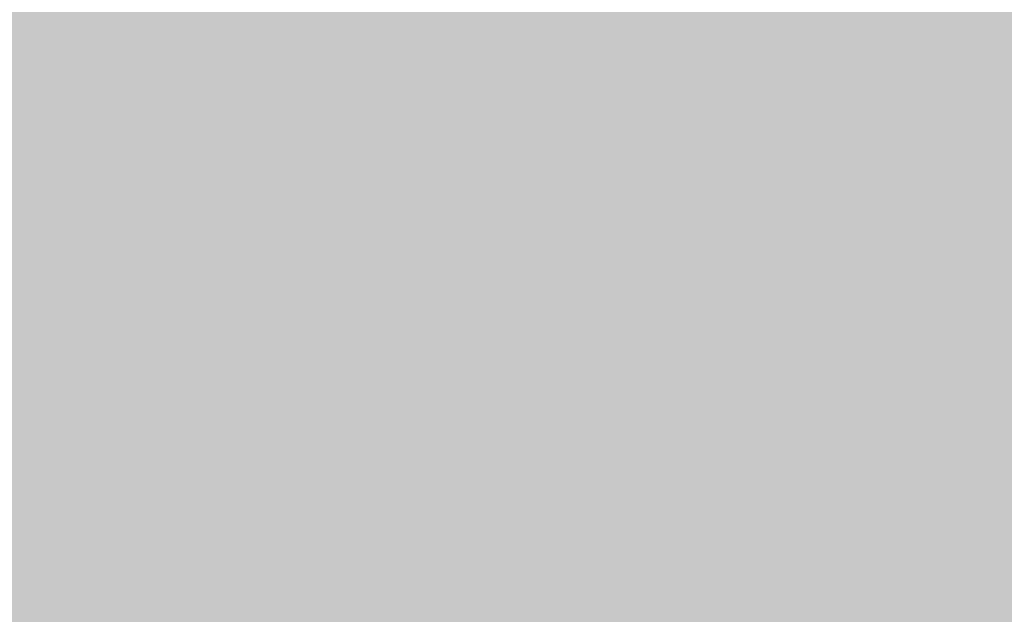
# Model space of a CAD drawing. Units: feet. Extents: x 3168 to 4724, y 827 to 1477.
# Tile 132 of 256: x 3300.858 to 3301.945, y 1098.344 to 1099.001. Entities that reach past the tile are written whole.
import ezdxf

# ---------------------------------------------------------------- set-up
doc = ezdxf.new("R2010")
doc.units = ezdxf.units.FT
doc.layers.add('A-ELEV', color=7, linetype='Continuous', lineweight=35)
doc.layers.add('A-ELEV-PATT', color=8, linetype='Continuous', lineweight=13)

msp = doc.modelspace()

# ---------------------------------------------------------------- hatches: boundary and pattern name
at = {"layer": 'A-ELEV-PATT'}
h = msp.add_hatch(color=256, dxfattribs=at)
h.dxf.hatch_style = 1
edge = h.paths.add_edge_path()
edge.add_ellipse((3552.9058, 979.2201), major_axis=(36.7449, 0), ratio=0.4848485, start_angle=0, end_angle=360)
edge = h.paths.add_edge_path()
edge.add_ellipse((3559.8916, 929.2523), major_axis=(36.7449, 0), ratio=0.4848485, start_angle=0, end_angle=360)
edge = h.paths.add_edge_path()
edge.add_line((3299.3168, 1198.6061), (3479.9167, 1198.6061))
edge.add_line((3479.9167, 1198.6061), (3479.9167, 1209.8686))
edge.add_spline(control_points=[(3479.9167, 1209.8686), (3464.3012, 1209.8686), (3448.6856, 1209.8686), (3410.9491, 1209.8686), (3388.8282, 1209.8686), (3355.6469, 1209.8686), (3344.5864, 1209.8686), (3327.9957, 1209.8686), (3322.4655, 1209.8686), (3314.1702, 1209.8686), (3311.4051, 1209.8686), (3307.2574, 1209.8686), (3305.8748, 1209.8686), (3303.801, 1209.8686), (3303.1097, 1209.8686), (3302.0728, 1209.8686), (3301.7272, 1209.8686), (3301.2087, 1209.8686), (3301.0359, 1209.8686), (3300.7767, 1209.8686), (3300.6903, 1209.8686), (3300.5606, 1209.8686), (3300.5174, 1209.8686), (3300.4526, 1209.8686), (3300.431, 1209.8686), (3300.3986, 1209.8686), (3300.3878, 1209.8686), (3300.3662, 1209.8686), (3300.3457, 1209.8686), (3300.3455, 1209.8686), (3300.3455, 1209.8686), (3300.3433, 1209.8686), (3300.3411, 1209.8686), (3300.3379, 1209.8686), (3300.3368, 1209.8686), (3300.3339, 1209.8686), (3300.3321, 1209.8686), (3300.3255, 1209.8686), (3300.3207, 1209.8686), (3300.3109, 1209.8686), (3300.306, 1209.8686), (3300.2905, 1209.8686), (3300.28, 1209.8686), (3300.2324, 1209.8688), (3300.1953, 1209.869), (3299.9511, 1209.8706), (3299.7448, 1209.8743), (3299.4368, 1209.8833), (3299.3344, 1209.8868), (3299.1811, 1209.8929), (3299.13, 1209.8951), (3298.6522, 1209.9168), (3298.2295, 1209.9457), (3297.6016, 1210.0024), (3297.3934, 1210.0235), (3297.0827, 1210.0583), (3296.9793, 1210.0705), (3296.293, 1210.1549), (3295.7181, 1210.2434), (3294.8687, 1210.3989), (3294.5877, 1210.4545), (3294.1693, 1210.5433), (3294.0304, 1210.5739), (3291.7071, 1211.1012), (3289.6536, 1211.8134), (3285.7763, 1213.564), (3283.9514, 1214.6035), (3280.5122, 1216.9801), (3278.8972, 1218.3176), (3276.3799, 1220.8295), (3275.416, 1221.9177), (3274.0393, 1223.7077), (3273.581, 1224.3495), (3273.1432, 1225.0163)], knot_values=[39.119033, 39.119033, 39.119033, 39.119033, 39.286353, 39.286353, 39.523379, 39.523379, 39.641892, 39.641892, 39.701148, 39.701148, 39.730777, 39.730777, 39.745591, 39.745591, 39.752998, 39.752998, 39.756701, 39.756701, 39.758553, 39.758553, 39.759479, 39.759479, 39.759942, 39.759942, 39.760173, 39.760173, 39.760289, 39.760289, 39.760405, 39.760405, 39.760463, 39.760463, 39.763389, 39.763389, 39.764851, 39.764851, 39.767304, 39.767304, 39.773825, 39.773825, 39.78057, 39.78057, 39.79477, 39.79477, 39.845194, 39.845194, 40.126715, 40.126715, 40.267476, 40.267476, 40.337856, 40.337856, 40.927023, 40.927023, 41.221606, 41.221606, 41.368898, 41.368898, 42.202622, 42.202622, 42.619485, 42.619485, 42.827916, 42.827916, 46.118323, 46.118323, 49.408731, 49.408731, 52.699139, 52.699139, 54.927489, 54.927489, 56.104228, 56.104228, 56.104228, 56.104228], weights=[1, 1, 1, 1, 1, 1, 1, 1, 1, 1, 1, 1, 1, 1, 1, 1, 1, 1, 1, 1, 1, 1, 1, 1, 1, 1, 1, 1, 1, 1, 1, 1, 1, 1, 1, 1, 1, 1, 1, 1, 1, 1, 1, 1, 1, 1, 1, 1, 1, 1, 1, 1, 1, 1, 1, 1, 1, 1, 1, 1, 1, 1, 1, 1, 1, 1, 1, 1, 1, 1, 1, 1, 1, 1], degree=3, periodic=0)
edge.add_line((3273.1432, 1225.0163), (3273.1432, 1099.0163))
edge.add_line((3273.1432, 1099.0163), (3299.3168, 1099.0163))
edge.add_line((3299.3168, 1099.0163), (3299.3168, 1198.6061))
edge = h.paths.add_edge_path()
edge.add_line((3304.7584, 1324.1581), (3479.9167, 1324.1581))
edge.add_line((3479.9167, 1324.1581), (3479.9167, 1335.7146))
edge.add_line((3479.9167, 1335.7146), (3269.1616, 1335.7146))
edge.add_spline(control_points=[(3269.1616, 1335.7146), (3264.0242, 1335.7146), (3258.3641, 1328.9582), (3259.2643, 1323.9003)], knot_values=[0, 0, 0, 0, 15.412191, 15.412191, 15.412191, 15.412191], degree=3, periodic=0)
edge.add_line((3259.2643, 1323.9003), (3265.5168, 1288.7691))
edge.add_line((3265.5168, 1288.7691), (3275.2651, 1261.5456))
edge.add_line((3275.2651, 1261.5456), (3304.7584, 1261.5456))
edge.add_line((3304.7584, 1261.5456), (3304.7584, 1324.1581))
h = msp.add_hatch(color=256, dxfattribs=at)
h.dxf.hatch_style = 1
h.paths.add_polyline_path([(3384.5252, 1099.0163), (3335.0292, 1099.0163), (3299.3168, 1099.0163), (3273.1432, 1099.0163), (3217.5654, 1099.0163), (3168.0693, 827.1163), (3335.0292, 827.1163)])

# ---------------------------------------------------------------- linework, layer by layer
at = {"layer": 'A-ELEV'}
msp.add_open_spline([(3808.5202, 1099.0163), (3808.5202, 1141.4132), (3808.5202, 1183.8102), (3808.5202, 1226.6353), (3808.5202, 1227.0636), (3808.5202, 1227.4918), (3811.4919, 1248.9947), (3814.4635, 1270.4975), (3817.4652, 1292.2176), (3817.4952, 1292.4348), (3817.5253, 1292.652), (3817.5728, 1310.1067), (3817.6203, 1327.5615), (3817.6679, 1345.0163), (3817.6679, 1345.458), (3817.6679, 1345.8996), (3817.6679, 1346.456), (3817.6679, 1346.5708), (3817.6679, 1346.7529), (3817.6679, 1346.8201), (3817.6679, 1346.9349), (3817.6679, 1346.9823), (3817.6679, 1347.0386), (3817.6679, 1347.0474), (3817.6679, 1347.0737), (3817.6679, 1347.0593), (3817.6679, 1347.0615), (3817.6679, 1347.0627), (3817.6679, 1347.066), (3817.6679, 1347.0683), (3817.6679, 1347.075), (3817.6679, 1347.0795), (3817.6678, 1347.0929), (3817.6678, 1347.1019), (3817.6678, 1347.1288), (3817.6677, 1347.1467), (3817.6674, 1347.2004), (3817.6672, 1347.2362), (3817.6661, 1347.3434), (3817.665, 1347.4147), (3817.6608, 1347.6281), (3817.6566, 1347.7697), (3817.64, 1348.1925), (3817.6235, 1348.4716), (3817.5591, 1349.3001), (3817.4961, 1349.8406), (3817.2554, 1351.4242), (3817.0263, 1352.4288), (3816.3069, 1354.8889), (3815.7437, 1356.2687), (3814.464, 1358.8192), (3813.7464, 1359.991), (3812.1958, 1362.1723), (3811.3622, 1363.1821), (3809.5888, 1365.069), (3808.6488, 1365.9461), (3806.6543, 1367.5796), (3805.5997, 1368.3362), (3803.3529, 1369.7223), (3802.1605, 1370.3524), (3799.6008, 1371.4536), (3798.2327, 1371.9255), (3795.2801, 1372.6346), (3793.6931, 1372.8721), (3791.8694, 1372.9265), (3791.7409, 1372.9292), (3791.3534, 1372.9341), (3791.0927, 1372.9329), (3790.3041, 1372.9151), (3789.7695, 1372.8842), (3789.2092, 1372.8302), (3789.1906, 1372.8284), (3789.1349, 1372.8229), (3789.0977, 1372.8191), (3789.0484, 1372.814), (3789.0364, 1372.8127), (3789.0003, 1372.8089), (3788.9761, 1372.8063), (3788.9494, 1372.8034), (3788.9468, 1372.8031), (3788.9426, 1372.8027), (3788.941, 1372.8025), (3788.9386, 1372.8022), (3788.9378, 1372.8021), (3788.9354, 1372.8019), (3788.8675, 1372.7944), (3788.7569, 1372.7822), (3788.7015, 1372.7761), (3788.5355, 1372.7579), (3788.4249, 1372.7457), (3788.0929, 1372.7092), (3787.8715, 1372.6848), (3787.2075, 1372.6118), (3786.7648, 1372.5631), (3785.4368, 1372.417), (3784.5515, 1372.3196), (3781.8954, 1372.0274), (3780.1247, 1371.8327), (3774.8126, 1371.2483), (3771.2713, 1370.8587), (3760.6471, 1369.69), (3753.5643, 1368.9109), (3732.316, 1366.5735), (3718.1504, 1365.0152), (3694.0068, 1362.3593), (3684.0287, 1361.2617), (3674.0506, 1360.1641), (3664.6007, 1360.1641), (3655.1508, 1360.1641), (3626.8011, 1360.1641), (3607.9013, 1360.1641), (3551.2019, 1360.1641), (3513.4023, 1360.1641), (3467.7252, 1360.1641), (3459.8476, 1360.1641), (3436.2149, 1360.1641), (3420.4597, 1360.1641), (3373.1943, 1360.1641), (3341.6839, 1360.1641), (3302.8482, 1360.1641), (3295.5227, 1360.1641), (3286.0383, 1360.1641), (3283.8794, 1360.1641), (3277.4026, 1360.1641), (3273.0848, 1360.1641), (3267.7329, 1360.1641), (3266.6988, 1360.1641), (3263.5965, 1360.1641), (3261.5284, 1360.1641), (3259.2369, 1360.1641), (3259.0137, 1360.1641), (3258.344, 1360.1641), (3257.8975, 1360.1641), (3257.431, 1360.1641), (3257.411, 1360.1641), (3257.3706, 1360.1641), (3257.3755, 1360.1641), (3257.3746, 1360.1641), (3257.3739, 1360.1641), (3257.372, 1360.1641), (3257.3706, 1360.1641), (3257.3667, 1360.1641), (3257.364, 1360.1641), (3257.3561, 1360.1641), (3257.3508, 1360.164), (3257.335, 1360.164), (3257.3244, 1360.164), (3257.2928, 1360.1639), (3257.2717, 1360.1638), (3257.2084, 1360.1634), (3257.1663, 1360.163), (3257.0402, 1360.1614), (3256.9563, 1360.1598), (3256.7055, 1360.1534), (3256.5392, 1360.147), (3256.0436, 1360.1219), (3255.7173, 1360.0971), (3254.7524, 1360.0005), (3254.128, 1359.9065), (3252.1801, 1359.5253), (3250.9416, 1359.144), (3248.6702, 1358.2433), (3247.6357, 1357.7238), (3245.7326, 1356.6035), (3244.8634, 1356.0021), (3243.2531, 1354.7429), (3242.512, 1354.0847), (3240.7511, 1352.3448), (3239.801, 1351.2296), (3238.0878, 1348.8724), (3237.3247, 1347.6304), (3235.9825, 1344.9716), (3235.4022, 1343.5549), (3234.5911, 1340.8155), (3234.3109, 1339.5435), (3233.9765, 1336.8026), (3233.9221, 1335.3309), (3234.1489, 1332.5913), (3234.3495, 1331.3672), (3234.7199, 1329.9994), (3234.7524, 1329.8834), (3234.8536, 1329.5348), (3234.9259, 1329.3017), (3235.0248, 1329.0026), (3235.0469, 1328.9369), (3235.0776, 1328.8472), (3235.0859, 1328.8232), (3235.1109, 1328.7511), (3235.1278, 1328.703), (3235.148, 1328.6462), (3235.1511, 1328.6376), (3235.1561, 1328.6235), (3235.1581, 1328.618), (3235.1602, 1328.612), (3235.1656, 1328.5969), (3235.1801, 1328.5565), (3235.1903, 1328.5281), (3235.2208, 1328.4429), (3235.2411, 1328.3862), (3235.3021, 1328.2159), (3235.3427, 1328.1023), (3235.4647, 1327.7617), (3235.546, 1327.5346), (3235.79, 1326.8534), (3235.9526, 1326.3992), (3236.4405, 1325.0367), (3236.7657, 1324.1284), (3237.7415, 1321.4034), (3238.392, 1319.5868), (3240.3435, 1314.1369), (3241.6445, 1310.5036), (3245.5476, 1299.6037), (3248.1496, 1292.3371), (3255.9557, 1270.5374), (3261.1598, 1256.0042), (3267.3876, 1238.612), (3268.4114, 1235.7529), (3269.5104, 1232.6839), (3269.5856, 1232.4739), (3269.7066, 1232.1359), (3269.7524, 1232.0079), (3269.8273, 1231.7987), (3269.8564, 1231.7176), (3269.9063, 1231.5781), (3269.9272, 1231.5198), (3269.9725, 1231.3934), (3269.9968, 1231.3254), (3270.0265, 1231.2425), (3270.0318, 1231.2277), (3270.0403, 1231.204), (3270.0392, 1231.207), (3270.0394, 1231.2066), (3270.0394, 1231.2064), (3270.0396, 1231.2058), (3270.0398, 1231.2055), (3270.0402, 1231.2043), (3270.0404, 1231.2036), (3270.0413, 1231.2013), (3270.0418, 1231.1998), (3270.0434, 1231.1953), (3270.0445, 1231.1922), (3270.0478, 1231.1832), (3270.0499, 1231.1771), (3270.0564, 1231.159), (3270.0608, 1231.147), (3270.0739, 1231.1108), (3270.0826, 1231.0867), (3270.1089, 1231.0144), (3270.1266, 1230.9663), (3270.1799, 1230.8225), (3270.2159, 1230.7269), (3270.3253, 1230.4415), (3270.4, 1230.2528), (3270.6292, 1229.6914), (3270.7889, 1229.3235), (3271.2865, 1228.2383), (3271.6431, 1227.5398), (3272.7759, 1225.5153), (3273.6142, 1224.2605), (3275.416, 1221.9177), (3276.3799, 1220.8295), (3278.8972, 1218.3176), (3280.5122, 1216.9801), (3283.9514, 1214.6035), (3285.7763, 1213.564), (3289.6536, 1211.8134), (3291.7071, 1211.1012), (3294.0304, 1210.5739), (3294.1693, 1210.5433), (3294.5877, 1210.4545), (3294.8687, 1210.3989), (3295.7181, 1210.2434), (3296.293, 1210.1549), (3296.9793, 1210.0705), (3297.0827, 1210.0583), (3297.3934, 1210.0235), (3297.6016, 1210.0024), (3298.2295, 1209.9457), (3298.6522, 1209.9168), (3299.13, 1209.8951), (3299.1811, 1209.8929), (3299.3344, 1209.8868), (3299.4368, 1209.8833), (3299.7448, 1209.8743), (3299.9511, 1209.8706), (3300.1953, 1209.869), (3300.2324, 1209.8688), (3300.28, 1209.8686), (3300.2905, 1209.8686), (3300.306, 1209.8686), (3300.3109, 1209.8686), (3300.3207, 1209.8686), (3300.3255, 1209.8686), (3300.3321, 1209.8686), (3300.3339, 1209.8686), (3300.3368, 1209.8686), (3300.3379, 1209.8686), (3300.3411, 1209.8686), (3300.3433, 1209.8686), (3300.3455, 1209.8686), (3300.3455, 1209.8686), (3300.3457, 1209.8686), (3300.3662, 1209.8686), (3300.3878, 1209.8686), (3300.3986, 1209.8686), (3300.431, 1209.8686), (3300.4526, 1209.8686), (3300.5174, 1209.8686), (3300.5606, 1209.8686), (3300.6903, 1209.8686), (3300.7767, 1209.8686), (3301.0359, 1209.8686), (3301.2087, 1209.8686), (3301.7272, 1209.8686), (3302.0728, 1209.8686), (3303.1097, 1209.8686), (3303.801, 1209.8686), (3305.8748, 1209.8686), (3307.2574, 1209.8686), (3311.4051, 1209.8686), (3314.1702, 1209.8686), (3322.4655, 1209.8686), (3327.9957, 1209.8686), (3344.5864, 1209.8686), (3355.6469, 1209.8686), (3388.8282, 1209.8686), (3410.9491, 1209.8686), (3477.3119, 1209.8686), (3521.5537, 1209.8686), (3566.8362, 1209.8686), (3567.8769, 1209.8686), (3570.999, 1209.8686), (3573.0804, 1209.8686), (3575.7814, 1209.8686), (3576.4009, 1209.8686), (3577.2958, 1209.8686), (3577.5712, 1209.8686), (3578.3971, 1209.8686), (3578.9478, 1209.8686), (3579.7565, 1209.8686), (3580.0145, 1209.8686), (3580.3427, 1209.8686), (3580.3269, 1209.8686), (3580.3272, 1209.8686), (3580.3273, 1209.8686), (3580.3278, 1209.8686), (3580.3281, 1209.8686), (3580.329, 1209.8686), (3580.3296, 1209.8686), (3580.3314, 1209.8686), (3580.3327, 1209.8686), (3580.3363, 1209.8686), (3580.3388, 1209.8686), (3580.3461, 1209.8686), (3580.351, 1209.8686), (3580.3657, 1209.8685), (3580.3754, 1209.8685), (3580.4048, 1209.8684), (3580.4244, 1209.8684), (3580.4832, 1209.8681), (3580.5224, 1209.8678), (3580.6404, 1209.8666), (3580.7192, 1209.8655), (3580.9563, 1209.8608), (3581.1152, 1209.8561), (3581.5942, 1209.8372), (3581.9164, 1209.8183), (3582.8899, 1209.7424), (3583.548, 1209.6662), (3585.5318, 1209.3606), (3586.8672, 1209.0539), (3589.4715, 1208.2525), (3590.7402, 1207.7579), (3591.9955, 1207.1588), (3592.0578, 1207.1287), (3592.2442, 1207.038), (3592.3677, 1206.9766), (3592.7353, 1206.7904), (3592.9768, 1206.6631), (3593.2445, 1206.5164), (3593.2747, 1206.4998), (3593.3651, 1206.4498), (3593.4251, 1206.4163), (3593.6043, 1206.3153), (3593.7227, 1206.2472), (3593.8572, 1206.1684), (3593.8744, 1206.1583), (3593.9257, 1206.128), (3593.9599, 1206.1078), (3594.0621, 1206.0469), (3594.1298, 1206.0061), (3594.2084, 1205.9582), (3594.2197, 1205.9513), (3594.2534, 1205.9307), (3594.2758, 1205.9169), (3594.343, 1205.8755), (3594.3876, 1205.8479), (3594.4336, 1205.819), (3594.4353, 1205.818), (3594.4402, 1205.8149), (3594.4435, 1205.8129), (3594.4471, 1205.8106), (3594.4475, 1205.8103), (3594.4487, 1205.8096), (3594.4495, 1205.8091), (3594.4504, 1205.8086), (3594.4505, 1205.8085), (3594.4506, 1205.8084), (3594.4674, 1205.7979), (3594.4933, 1205.7817), (3594.5062, 1205.7736), (3594.545, 1205.7492), (3594.5709, 1205.733), (3594.6485, 1205.6844), (3594.7002, 1205.652), (3594.8554, 1205.5547), (3594.9589, 1205.4898), (3595.2694, 1205.2953), (3595.4763, 1205.1656), (3596.0972, 1204.7765), (3596.5111, 1204.5171), (3597.7528, 1203.7388), (3598.5807, 1203.22), (3601.0642, 1201.6636), (3602.7198, 1200.6259), (3607.6868, 1197.513), (3610.9981, 1195.4377), (3620.932, 1189.2119), (3627.5546, 1185.0614), (3647.4225, 1172.6097), (3660.6678, 1164.3086), (3700.4035, 1139.4053), (3726.894, 1122.8031), (3757.2057, 1103.8061), (3761.027, 1101.4112), (3764.8482, 1099.0163), (3745.3283, 1099.0163), (3725.8083, 1099.0163), (3706.2884, 1099.0163), (3706.2884, 1108.4532), (3706.2884, 1117.8902), (3706.2884, 1127.3271), (3710.7508, 1127.3271), (3715.2131, 1127.3271), (3719.6755, 1127.3271)], degree=3, knots=[0, 0, 0, 0, 0.982037, 0.982037, 0.991957, 0.991957, 0.991957, 1.966522, 1.966522, 1.976367, 1.976367, 1.976367, 2.976367, 2.976367, 2.976367, 3.00169, 3.00169, 3.008272, 3.008272, 3.012129, 3.012129, 3.014851, 3.014851, 3.015353, 3.015353, 3.016359, 3.016359, 3.017365, 3.017365, 3.019376, 3.019376, 3.023398, 3.023398, 3.031442, 3.031442, 3.047531, 3.047531, 3.079708, 3.079708, 3.144063, 3.144063, 3.272772, 3.272772, 3.53019, 3.53019, 4.045026, 4.045026, 5.074698, 5.074698, 6.700878, 6.700878, 8.327058, 8.327058, 9.953238, 9.953238, 11.579418, 11.579418, 13.205598, 13.205598, 14.831778, 14.831778, 16.457958, 16.457958, 18.084138, 18.084138, 18.206872, 18.206872, 18.45234, 18.45234, 18.943275, 18.943275, 18.960093, 18.960093, 18.993729, 18.993729, 19.00461, 19.00461, 19.026374, 19.026374, 19.028737, 19.028737, 19.03018, 19.03018, 19.030897, 19.030897, 19.032332, 19.032332, 19.033766, 19.033766, 19.036636, 19.036636, 19.042374, 19.042374, 19.053851, 19.053851, 19.076805, 19.076805, 19.122714, 19.122714, 19.21453, 19.21453, 19.398163, 19.398163, 19.765429, 19.765429, 20.024128, 20.024128, 20.024128, 20.092031, 20.092031, 20.227836, 20.227836, 20.499446, 20.499446, 20.556051, 20.556051, 20.66926, 20.66926, 20.895678, 20.895678, 20.948316, 20.948316, 20.963829, 20.963829, 20.994855, 20.994855, 21.002285, 21.002285, 21.017146, 21.017146, 21.01875, 21.01875, 21.021959, 21.021959, 21.022102, 21.022102, 21.022249, 21.022249, 21.022708, 21.022708, 21.023627, 21.023627, 21.025464, 21.025464, 21.029138, 21.029138, 21.036486, 21.036486, 21.051183, 21.051183, 21.080575, 21.080575, 21.139361, 21.139361, 21.256932, 21.256932, 21.492073, 21.492073, 21.962356, 21.962356, 23.01002, 23.01002, 24.057684, 24.057684, 25.105348, 25.105348, 26.153011, 26.153011, 27.776787, 27.776787, 29.400562, 29.400562, 31.024337, 31.024337, 32.278801, 32.278801, 33.533265, 33.533265, 34.467568, 34.467568, 34.553971, 34.553971, 34.726776, 34.726776, 34.775309, 34.775309, 34.793079, 34.793079, 34.82862, 34.82862, 34.834979, 34.834979, 34.839039, 34.839039, 34.839411, 34.839411, 34.840285, 34.840285, 34.842034, 34.842034, 34.845531, 34.845531, 34.852525, 34.852525, 34.866512, 34.866512, 34.894488, 34.894488, 34.950439, 34.950439, 35.062342, 35.062342, 35.286147, 35.286147, 35.733758, 35.733758, 35.821815, 35.821815, 35.828283, 35.828283, 35.832225, 35.832225, 35.834724, 35.834724, 35.836521, 35.836521, 35.838617, 35.838617, 35.839073, 35.839073, 35.839345, 35.839345, 35.839617, 35.839617, 35.840161, 35.840161, 35.841249, 35.841249, 35.843425, 35.843425, 35.847778, 35.847778, 35.856482, 35.856482, 35.873891, 35.873891, 35.908709, 35.908709, 35.978345, 35.978345, 36.117617, 36.117617, 36.396161, 36.396161, 36.953248, 36.953248, 38.067423, 38.067423, 40.295772, 40.295772, 42.524122, 42.524122, 45.81453, 45.81453, 49.104937, 49.104937, 52.395345, 52.395345, 52.603776, 52.603776, 53.020639, 53.020639, 53.854363, 53.854363, 54.001655, 54.001655, 54.296238, 54.296238, 54.885405, 54.885405, 54.955785, 54.955785, 55.096546, 55.096546, 55.378067, 55.378067, 55.42849, 55.42849, 55.442691, 55.442691, 55.449436, 55.449436, 55.455957, 55.455957, 55.458409, 55.458409, 55.459872, 55.459872, 55.462798, 55.462798, 55.462856, 55.462856, 55.462972, 55.462972, 55.463088, 55.463088, 55.463319, 55.463319, 55.463782, 55.463782, 55.464708, 55.464708, 55.46656, 55.46656, 55.470263, 55.470263, 55.47767, 55.47767, 55.492484, 55.492484, 55.522112, 55.522112, 55.581369, 55.581369, 55.699882, 55.699882, 55.936907, 55.936907, 56.410959, 56.410959, 56.42211, 56.42211, 56.444413, 56.444413, 56.451051, 56.451051, 56.454001, 56.454001, 56.459901, 56.459901, 56.462666, 56.462666, 56.463418, 56.463418, 56.464171, 56.464171, 56.465675, 56.465675, 56.468684, 56.468684, 56.474702, 56.474702, 56.486738, 56.486738, 56.51081, 56.51081, 56.558955, 56.558955, 56.655243, 56.655243, 56.847821, 56.847821, 57.232975, 57.232975, 58.003284, 58.003284, 59.543901, 59.543901, 62.625137, 62.625137, 68.787607, 68.787607, 74.950078, 74.950078, 75.27336, 75.27336, 75.919923, 75.919923, 77.213051, 77.213051, 77.377769, 77.377769, 77.707206, 77.707206, 78.366079, 78.366079, 78.462532, 78.462532, 78.655436, 78.655436, 79.041245, 79.041245, 79.105735, 79.105735, 79.234714, 79.234714, 79.492672, 79.492672, 79.502197, 79.502197, 79.521249, 79.521249, 79.523534, 79.523534, 79.528103, 79.528103, 79.528682, 79.528682, 79.528885, 79.528885, 79.529089, 79.529089, 79.529495, 79.529495, 79.530308, 79.530308, 79.531935, 79.531935, 79.535187, 79.535187, 79.541693, 79.541693, 79.554704, 79.554704, 79.580725, 79.580725, 79.632769, 79.632769, 79.736856, 79.736856, 79.94503, 79.94503, 80.361377, 80.361377, 80.421435, 80.421435, 80.421435, 81.421435, 81.421435, 81.421435, 82.421435, 82.421435, 82.421435, 83.421435, 83.421435, 83.421435, 83.421435], dxfattribs=at)

doc.saveas('drawing.dxf')
